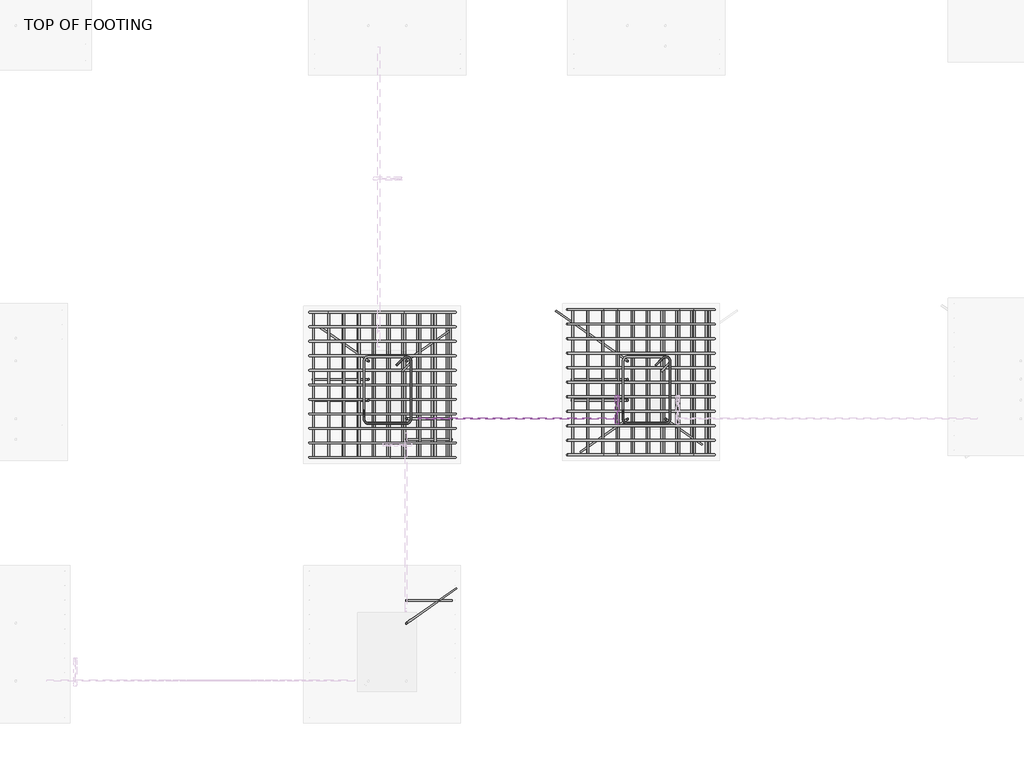
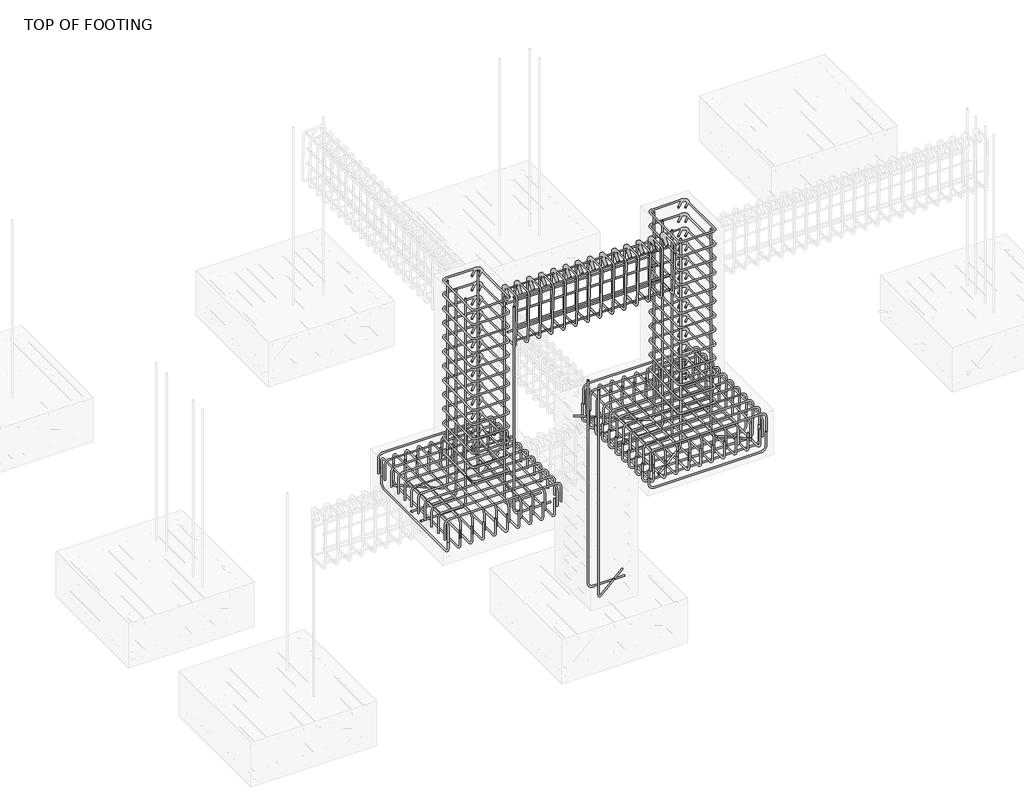
# One storey, part 4 of 17: 24 reinforcing bars.
"""IFC4 building model written with IfcOpenShell, lengths in millimetres."""

from ifc_helpers import new_model, si_unit, point, frame, origin, place, context, project, spatial, polyline, circle_curve, trimmed, segment, composite_curve, source, transform, mapped, element, save
from ifc_brep_helpers import swept_disk

model = new_model("IFC4")

# Units and contexts
model_context = context("Model", 3, world=origin())
ifc_project = project(units=[si_unit("LENGTHUNIT", "METRE", prefix="MILLI")], contexts=[model_context])

# Site, building, storey
site = spatial("IfcSite", under=ifc_project)
building = spatial("IfcBuilding", under=site)
storey = spatial("IfcBuildingStorey", under=building, Name="TOP OF FOOTING", Elevation=-1828.8)

# Reinforcing bars
placement = place(None, origin())
reinforcing_bar_shape = source(origin(), model_context, "Body", "SolidModel", [
    swept_disk(composite_curve([segment(polyline([(-908.0711351, -340.8742842, -2058.517229), (-908.0711351, -340.8742842, -1911.217229)]), True, "CONTINUOUS"), segment(trimmed(circle_curve(frame((-861.7211351, -340.8742842, -1911.217229), z_axis=(0.0, 1.0, 0.0), x_axis=(-46.35000000000002, 0.0, 0.0)), 46.35), [point((-908.0711351, -340.8742842, -1911.217229))], [point((-861.7211351, -340.8742842, -1864.867229))], True, "CARTESIAN"), True, "CONTINUOUS"), segment(polyline([(-861.7211351, -340.8742842, -1864.867229), (156.8352514, -340.8742842, -1864.867229)]), True, "CONTINUOUS"), segment(trimmed(circle_curve(frame((156.8352514, -340.8742842, -1911.217229), z_axis=(0.0, 1.0, 0.0), x_axis=(0.0, 0.0, 46.350000000000136)), 46.35), [point((156.8352514, -340.8742842, -1864.867229))], [point((203.1852514, -340.8742842, -1911.217229))], True, "CARTESIAN"), True, "CONTINUOUS"), segment(polyline([(203.1852514, -340.8742842, -1911.217229), (203.1852514, -340.8742842, -2058.517229)]), True, "CONTINUOUS")], self_intersect=False), 6.35),
])
element("IfcReinforcingBar", 1, at=placement, inside=storey, context=model_context, shape_type="MappedRepresentation", body=[
    mapped(reinforcing_bar_shape, transform((0.0, 0.0, 0.0), x_axis=(1.0, 0.0, 0.0), y_axis=(0.0, 1.0, 0.0), z_axis=(0.0, 0.0, 1.0))),
    mapped(reinforcing_bar_shape, transform((0.0, -110.73, 0.0), x_axis=(1.0, 0.0, 0.0), y_axis=(0.0, 1.0, 0.0), z_axis=(0.0, 0.0, 1.0))),
    mapped(reinforcing_bar_shape, transform((0.0, -221.46, 0.0), x_axis=(1.0, 0.0, 0.0), y_axis=(0.0, 1.0, 0.0), z_axis=(0.0, 0.0, 1.0))),
    mapped(reinforcing_bar_shape, transform((0.0, -332.19, 0.0), x_axis=(1.0, 0.0, 0.0), y_axis=(0.0, 1.0, 0.0), z_axis=(0.0, 0.0, 1.0))),
    mapped(reinforcing_bar_shape, transform((0.0, -442.92, 0.0), x_axis=(1.0, 0.0, 0.0), y_axis=(0.0, 1.0, 0.0), z_axis=(0.0, 0.0, 1.0))),
    mapped(reinforcing_bar_shape, transform((0.0, -553.65, 0.0), x_axis=(1.0, 0.0, 0.0), y_axis=(0.0, 1.0, 0.0), z_axis=(0.0, 0.0, 1.0))),
    mapped(reinforcing_bar_shape, transform((0.0, -664.38, 0.0), x_axis=(1.0, 0.0, 0.0), y_axis=(0.0, 1.0, 0.0), z_axis=(0.0, 0.0, 1.0))),
    mapped(reinforcing_bar_shape, transform((0.0, -775.11, 0.0), x_axis=(1.0, 0.0, 0.0), y_axis=(0.0, 1.0, 0.0), z_axis=(0.0, 0.0, 1.0))),
    mapped(reinforcing_bar_shape, transform((0.0, -885.84, 0.0), x_axis=(1.0, 0.0, 0.0), y_axis=(0.0, 1.0, 0.0), z_axis=(0.0, 0.0, 1.0))),
    mapped(reinforcing_bar_shape, transform((0.0, -996.57, 0.0), x_axis=(1.0, 0.0, 0.0), y_axis=(0.0, 1.0, 0.0), z_axis=(0.0, 0.0, 1.0))),
    mapped(reinforcing_bar_shape, transform((0.0, -1107.3, 0.0), x_axis=(1.0, 0.0, 0.0), y_axis=(0.0, 1.0, 0.0), z_axis=(0.0, 0.0, 1.0))),
])
reinforcing_bar_2_shape = source(origin(), model_context, "Body", "SolidModel", [
    swept_disk(composite_curve([segment(polyline([(166.1935463, -340.8742842, -2093.0974099), (166.1935463, -340.8742842, -1945.7974099)]), True, "CONTINUOUS"), segment(trimmed(circle_curve(frame((166.1935463, -387.2242842, -1945.7974099), z_axis=(1.0, 0.0, 0.0), x_axis=(0.0, 46.35000000000002, 0.0)), 46.35), [point((166.1935463, -340.8742842, -1945.7974099))], [point((166.1935463, -387.2242842, -1899.4474099))], True, "CARTESIAN"), True, "CONTINUOUS"), segment(polyline([(166.1935463, -387.2242842, -1899.4474099), (166.1935463, -1401.8242842, -1899.4474099)]), True, "CONTINUOUS"), segment(trimmed(circle_curve(frame((166.1935463, -1401.8242842, -1945.7974099), z_axis=(1.0, 0.0, 0.0), x_axis=(0.0, 0.0, 46.350000000000136)), 46.35), [point((166.1935463, -1401.8242842, -1899.4474099))], [point((166.1935463, -1448.1742842, -1945.7974099))], True, "CARTESIAN"), True, "CONTINUOUS"), segment(polyline([(166.1935463, -1448.1742842, -1945.7974099), (166.1935463, -1448.1742842, -2093.0974099)]), True, "CONTINUOUS")], self_intersect=False), 6.35),
])
element("IfcReinforcingBar", 2, at=placement, inside=storey, context=model_context, shape_type="MappedRepresentation", body=[
    mapped(reinforcing_bar_2_shape, transform((0.0, 0.0, 0.0), x_axis=(1.0, 0.0, 0.0), y_axis=(0.0, 1.0, 0.0), z_axis=(0.0, 0.0, 1.0))),
    mapped(reinforcing_bar_2_shape, transform((-115.9606781, 0.0, 0.0), x_axis=(1.0, 0.0, 0.0), y_axis=(0.0, 1.0, 0.0), z_axis=(0.0, 0.0, 1.0))),
    mapped(reinforcing_bar_2_shape, transform((-231.9213561, 0.0, 0.0), x_axis=(1.0, 0.0, 0.0), y_axis=(0.0, 1.0, 0.0), z_axis=(0.0, 0.0, 1.0))),
    mapped(reinforcing_bar_2_shape, transform((-347.8820342, 0.0, 0.0), x_axis=(1.0, 0.0, 0.0), y_axis=(0.0, 1.0, 0.0), z_axis=(0.0, 0.0, 1.0))),
    mapped(reinforcing_bar_2_shape, transform((-463.8427123, 0.0, 0.0), x_axis=(1.0, 0.0, 0.0), y_axis=(0.0, 1.0, 0.0), z_axis=(0.0, 0.0, 1.0))),
    mapped(reinforcing_bar_2_shape, transform((-579.8033904, 0.0, 0.0), x_axis=(1.0, 0.0, 0.0), y_axis=(0.0, 1.0, 0.0), z_axis=(0.0, 0.0, 1.0))),
    mapped(reinforcing_bar_2_shape, transform((-695.7640684, 0.0, 0.0), x_axis=(1.0, 0.0, 0.0), y_axis=(0.0, 1.0, 0.0), z_axis=(0.0, 0.0, 1.0))),
    mapped(reinforcing_bar_2_shape, transform((-811.7247465, 0.0, 0.0), x_axis=(1.0, 0.0, 0.0), y_axis=(0.0, 1.0, 0.0), z_axis=(0.0, 0.0, 1.0))),
    mapped(reinforcing_bar_2_shape, transform((-927.6854246, 0.0, 0.0), x_axis=(1.0, 0.0, 0.0), y_axis=(0.0, 1.0, 0.0), z_axis=(0.0, 0.0, 1.0))),
    mapped(reinforcing_bar_2_shape, transform((-1043.6461027, 0.0, 0.0), x_axis=(1.0, 0.0, 0.0), y_axis=(0.0, 1.0, 0.0), z_axis=(0.0, 0.0, 1.0))),
])
reinforcing_bar_3_shape = source(origin(), model_context, "Body", "SolidModel", [
    swept_disk(composite_curve([segment(polyline([(-877.4525564, -340.8742842, -2009.4698822), (-877.4525564, -340.8742842, -2156.7698822)]), True, "CONTINUOUS"), segment(trimmed(circle_curve(frame((-877.4525564, -387.2242842, -2156.7698822), z_axis=(-1.0, 0.0, 0.0), x_axis=(0.0, 46.35000000000002, 0.0)), 46.35), [point((-877.4525564, -340.8742842, -2156.7698822))], [point((-877.4525564, -387.2242842, -2203.1198822))], True, "CARTESIAN"), True, "CONTINUOUS"), segment(polyline([(-877.4525564, -387.2242842, -2203.1198822), (-877.4525564, -1401.8242842, -2203.1198822)]), True, "CONTINUOUS"), segment(trimmed(circle_curve(frame((-877.4525564, -1401.8242842, -2156.7698822), z_axis=(-1.0, 0.0, 0.0), x_axis=(0.0, 0.0, -46.34999999999991)), 46.35), [point((-877.4525564, -1401.8242842, -2203.1198822))], [point((-877.4525564, -1448.1742842, -2156.7698822))], True, "CARTESIAN"), True, "CONTINUOUS"), segment(polyline([(-877.4525564, -1448.1742842, -2156.7698822), (-877.4525564, -1448.1742842, -2009.4698822)]), True, "CONTINUOUS")], self_intersect=False), 6.35),
])
element("IfcReinforcingBar", 3, at=placement, inside=storey, context=model_context, shape_type="MappedRepresentation", body=[
    mapped(reinforcing_bar_3_shape, transform((0.0, 0.0, 0.0), x_axis=(1.0, 0.0, 0.0), y_axis=(0.0, 1.0, 0.0), z_axis=(0.0, 0.0, 1.0))),
    mapped(reinforcing_bar_3_shape, transform((113.1523491, 0.0, 0.0), x_axis=(1.0, 0.0, 0.0), y_axis=(0.0, 1.0, 0.0), z_axis=(0.0, 0.0, 1.0))),
    mapped(reinforcing_bar_3_shape, transform((226.3046983, 0.0, 0.0), x_axis=(1.0, 0.0, 0.0), y_axis=(0.0, 1.0, 0.0), z_axis=(0.0, 0.0, 1.0))),
    mapped(reinforcing_bar_3_shape, transform((339.4570474, 0.0, 0.0), x_axis=(1.0, 0.0, 0.0), y_axis=(0.0, 1.0, 0.0), z_axis=(0.0, 0.0, 1.0))),
    mapped(reinforcing_bar_3_shape, transform((452.6093966, 0.0, 0.0), x_axis=(1.0, 0.0, 0.0), y_axis=(0.0, 1.0, 0.0), z_axis=(0.0, 0.0, 1.0))),
    mapped(reinforcing_bar_3_shape, transform((565.7617457, 0.0, 0.0), x_axis=(1.0, 0.0, 0.0), y_axis=(0.0, 1.0, 0.0), z_axis=(0.0, 0.0, 1.0))),
    mapped(reinforcing_bar_3_shape, transform((678.9140949, 0.0, 0.0), x_axis=(1.0, 0.0, 0.0), y_axis=(0.0, 1.0, 0.0), z_axis=(0.0, 0.0, 1.0))),
    mapped(reinforcing_bar_3_shape, transform((792.066444, 0.0, 0.0), x_axis=(1.0, 0.0, 0.0), y_axis=(0.0, 1.0, 0.0), z_axis=(0.0, 0.0, 1.0))),
    mapped(reinforcing_bar_3_shape, transform((905.2187932, 0.0, 0.0), x_axis=(1.0, 0.0, 0.0), y_axis=(0.0, 1.0, 0.0), z_axis=(0.0, 0.0, 1.0))),
    mapped(reinforcing_bar_3_shape, transform((1018.3711423, 0.0, 0.0), x_axis=(1.0, 0.0, 0.0), y_axis=(0.0, 1.0, 0.0), z_axis=(0.0, 0.0, 1.0))),
])
reinforcing_bar_4_shape = source(origin(), model_context, "Body", "SolidModel", [
    swept_disk(composite_curve([segment(polyline([(2175.7588658, -320.8742842, -2051.4362487), (2175.7588658, -320.8742842, -2198.7362487)]), True, "CONTINUOUS"), segment(trimmed(circle_curve(frame((2129.4088658, -320.8742842, -2198.7362487), z_axis=(0.0, 1.0, 0.0), x_axis=(46.34999999999991, 0.0, 0.0)), 46.35), [point((2175.7588658, -320.8742842, -2198.7362487))], [point((2129.4088658, -320.8742842, -2245.0862487))], True, "CARTESIAN"), True, "CONTINUOUS"), segment(polyline([(2129.4088658, -320.8742842, -2245.0862487), (1104.0910413, -320.8742842, -2245.0862487)]), True, "CONTINUOUS"), segment(trimmed(circle_curve(frame((1104.0910413, -320.8742842, -2198.7362487), z_axis=(0.0, 1.0, 0.0), x_axis=(0.0, 0.0, -46.34999999999991)), 46.35), [point((1104.0910413, -320.8742842, -2245.0862487))], [point((1057.7410413, -320.8742842, -2198.7362487))], True, "CARTESIAN"), True, "CONTINUOUS"), segment(polyline([(1057.7410413, -320.8742842, -2198.7362487), (1057.7410413, -320.8742842, -2051.4362487)]), True, "CONTINUOUS")], self_intersect=False), 6.35),
])
element("IfcReinforcingBar", 4, at=placement, inside=storey, context=model_context, shape_type="MappedRepresentation", body=[
    mapped(reinforcing_bar_4_shape, transform((0.0, 0.0, 0.0), x_axis=(1.0, 0.0, 0.0), y_axis=(0.0, 1.0, 0.0), z_axis=(0.0, 0.0, 1.0))),
    mapped(reinforcing_bar_4_shape, transform((0.0, -110.73, 0.0), x_axis=(1.0, 0.0, 0.0), y_axis=(0.0, 1.0, 0.0), z_axis=(0.0, 0.0, 1.0))),
    mapped(reinforcing_bar_4_shape, transform((0.0, -221.46, 0.0), x_axis=(1.0, 0.0, 0.0), y_axis=(0.0, 1.0, 0.0), z_axis=(0.0, 0.0, 1.0))),
    mapped(reinforcing_bar_4_shape, transform((0.0, -332.19, 0.0), x_axis=(1.0, 0.0, 0.0), y_axis=(0.0, 1.0, 0.0), z_axis=(0.0, 0.0, 1.0))),
    mapped(reinforcing_bar_4_shape, transform((0.0, -442.92, 0.0), x_axis=(1.0, 0.0, 0.0), y_axis=(0.0, 1.0, 0.0), z_axis=(0.0, 0.0, 1.0))),
    mapped(reinforcing_bar_4_shape, transform((0.0, -553.65, 0.0), x_axis=(1.0, 0.0, 0.0), y_axis=(0.0, 1.0, 0.0), z_axis=(0.0, 0.0, 1.0))),
    mapped(reinforcing_bar_4_shape, transform((0.0, -664.38, 0.0), x_axis=(1.0, 0.0, 0.0), y_axis=(0.0, 1.0, 0.0), z_axis=(0.0, 0.0, 1.0))),
    mapped(reinforcing_bar_4_shape, transform((0.0, -775.11, 0.0), x_axis=(1.0, 0.0, 0.0), y_axis=(0.0, 1.0, 0.0), z_axis=(0.0, 0.0, 1.0))),
    mapped(reinforcing_bar_4_shape, transform((0.0, -885.84, 0.0), x_axis=(1.0, 0.0, 0.0), y_axis=(0.0, 1.0, 0.0), z_axis=(0.0, 0.0, 1.0))),
    mapped(reinforcing_bar_4_shape, transform((0.0, -996.57, 0.0), x_axis=(1.0, 0.0, 0.0), y_axis=(0.0, 1.0, 0.0), z_axis=(0.0, 0.0, 1.0))),
    mapped(reinforcing_bar_4_shape, transform((0.0, -1107.3, 0.0), x_axis=(1.0, 0.0, 0.0), y_axis=(0.0, 1.0, 0.0), z_axis=(0.0, 0.0, 1.0))),
])
reinforcing_bar_5_shape = source(origin(), model_context, "Body", "SolidModel", [
    swept_disk(composite_curve([segment(polyline([(1068.404705, -320.8742842, -2058.517229), (1068.404705, -320.8742842, -1911.217229)]), True, "CONTINUOUS"), segment(trimmed(circle_curve(frame((1114.754705, -320.8742842, -1911.217229), z_axis=(0.0, 1.0, 0.0), x_axis=(-46.350000000000136, 0.0, 0.0)), 46.35), [point((1068.404705, -320.8742842, -1911.217229))], [point((1114.754705, -320.8742842, -1864.867229))], True, "CARTESIAN"), True, "CONTINUOUS"), segment(polyline([(1114.754705, -320.8742842, -1864.867229), (2133.3110915, -320.8742842, -1864.867229)]), True, "CONTINUOUS"), segment(trimmed(circle_curve(frame((2133.3110915, -320.8742842, -1911.217229), z_axis=(0.0, 1.0, 0.0), x_axis=(0.0, 0.0, 46.350000000000136)), 46.35), [point((2133.3110915, -320.8742842, -1864.867229))], [point((2179.6610915, -320.8742842, -1911.217229))], True, "CARTESIAN"), True, "CONTINUOUS"), segment(polyline([(2179.6610915, -320.8742842, -1911.217229), (2179.6610915, -320.8742842, -2058.517229)]), True, "CONTINUOUS")], self_intersect=False), 6.35),
])
element("IfcReinforcingBar", 5, at=placement, inside=storey, context=model_context, shape_type="MappedRepresentation", body=[
    mapped(reinforcing_bar_5_shape, transform((0.0, 0.0, 0.0), x_axis=(1.0, 0.0, 0.0), y_axis=(0.0, 1.0, 0.0), z_axis=(0.0, 0.0, 1.0))),
    mapped(reinforcing_bar_5_shape, transform((0.0, -110.73, 0.0), x_axis=(1.0, 0.0, 0.0), y_axis=(0.0, 1.0, 0.0), z_axis=(0.0, 0.0, 1.0))),
    mapped(reinforcing_bar_5_shape, transform((0.0, -221.46, 0.0), x_axis=(1.0, 0.0, 0.0), y_axis=(0.0, 1.0, 0.0), z_axis=(0.0, 0.0, 1.0))),
    mapped(reinforcing_bar_5_shape, transform((0.0, -332.19, 0.0), x_axis=(1.0, 0.0, 0.0), y_axis=(0.0, 1.0, 0.0), z_axis=(0.0, 0.0, 1.0))),
    mapped(reinforcing_bar_5_shape, transform((0.0, -442.92, 0.0), x_axis=(1.0, 0.0, 0.0), y_axis=(0.0, 1.0, 0.0), z_axis=(0.0, 0.0, 1.0))),
    mapped(reinforcing_bar_5_shape, transform((0.0, -553.65, 0.0), x_axis=(1.0, 0.0, 0.0), y_axis=(0.0, 1.0, 0.0), z_axis=(0.0, 0.0, 1.0))),
    mapped(reinforcing_bar_5_shape, transform((0.0, -664.38, 0.0), x_axis=(1.0, 0.0, 0.0), y_axis=(0.0, 1.0, 0.0), z_axis=(0.0, 0.0, 1.0))),
    mapped(reinforcing_bar_5_shape, transform((0.0, -775.11, 0.0), x_axis=(1.0, 0.0, 0.0), y_axis=(0.0, 1.0, 0.0), z_axis=(0.0, 0.0, 1.0))),
    mapped(reinforcing_bar_5_shape, transform((0.0, -885.84, 0.0), x_axis=(1.0, 0.0, 0.0), y_axis=(0.0, 1.0, 0.0), z_axis=(0.0, 0.0, 1.0))),
    mapped(reinforcing_bar_5_shape, transform((0.0, -996.57, 0.0), x_axis=(1.0, 0.0, 0.0), y_axis=(0.0, 1.0, 0.0), z_axis=(0.0, 0.0, 1.0))),
    mapped(reinforcing_bar_5_shape, transform((0.0, -1107.3, 0.0), x_axis=(1.0, 0.0, 0.0), y_axis=(0.0, 1.0, 0.0), z_axis=(0.0, 0.0, 1.0))),
])
reinforcing_bar_6_shape = source(origin(), model_context, "Body", "SolidModel", [
    swept_disk(composite_curve([segment(polyline([(2142.6693864, -320.8742842, -2093.0974099), (2142.6693864, -320.8742842, -1945.7974099)]), True, "CONTINUOUS"), segment(trimmed(circle_curve(frame((2142.6693864, -367.2242842, -1945.7974099), z_axis=(1.0, 0.0, 0.0), x_axis=(0.0, 46.35000000000002, 0.0)), 46.35), [point((2142.6693864, -320.8742842, -1945.7974099))], [point((2142.6693864, -367.2242842, -1899.4474099))], True, "CARTESIAN"), True, "CONTINUOUS"), segment(polyline([(2142.6693864, -367.2242842, -1899.4474099), (2142.6693864, -1381.8242842, -1899.4474099)]), True, "CONTINUOUS"), segment(trimmed(circle_curve(frame((2142.6693864, -1381.8242842, -1945.7974099), z_axis=(1.0, 0.0, 0.0), x_axis=(0.0, 0.0, 46.350000000000136)), 46.35), [point((2142.6693864, -1381.8242842, -1899.4474099))], [point((2142.6693864, -1428.1742842, -1945.7974099))], True, "CARTESIAN"), True, "CONTINUOUS"), segment(polyline([(2142.6693864, -1428.1742842, -1945.7974099), (2142.6693864, -1428.1742842, -2093.0974099)]), True, "CONTINUOUS")], self_intersect=False), 6.35),
])
element("IfcReinforcingBar", 6, at=placement, inside=storey, context=model_context, shape_type="MappedRepresentation", body=[
    mapped(reinforcing_bar_6_shape, transform((0.0, 0.0, 0.0), x_axis=(1.0, 0.0, 0.0), y_axis=(0.0, 1.0, 0.0), z_axis=(0.0, 0.0, 1.0))),
    mapped(reinforcing_bar_6_shape, transform((-115.9606781, 0.0, 0.0), x_axis=(1.0, 0.0, 0.0), y_axis=(0.0, 1.0, 0.0), z_axis=(0.0, 0.0, 1.0))),
    mapped(reinforcing_bar_6_shape, transform((-231.9213561, 0.0, 0.0), x_axis=(1.0, 0.0, 0.0), y_axis=(0.0, 1.0, 0.0), z_axis=(0.0, 0.0, 1.0))),
    mapped(reinforcing_bar_6_shape, transform((-347.8820342, 0.0, 0.0), x_axis=(1.0, 0.0, 0.0), y_axis=(0.0, 1.0, 0.0), z_axis=(0.0, 0.0, 1.0))),
    mapped(reinforcing_bar_6_shape, transform((-463.8427123, 0.0, 0.0), x_axis=(1.0, 0.0, 0.0), y_axis=(0.0, 1.0, 0.0), z_axis=(0.0, 0.0, 1.0))),
    mapped(reinforcing_bar_6_shape, transform((-579.8033904, 0.0, 0.0), x_axis=(1.0, 0.0, 0.0), y_axis=(0.0, 1.0, 0.0), z_axis=(0.0, 0.0, 1.0))),
    mapped(reinforcing_bar_6_shape, transform((-695.7640684, 0.0, 0.0), x_axis=(1.0, 0.0, 0.0), y_axis=(0.0, 1.0, 0.0), z_axis=(0.0, 0.0, 1.0))),
    mapped(reinforcing_bar_6_shape, transform((-811.7247465, 0.0, 0.0), x_axis=(1.0, 0.0, 0.0), y_axis=(0.0, 1.0, 0.0), z_axis=(0.0, 0.0, 1.0))),
    mapped(reinforcing_bar_6_shape, transform((-927.6854246, 0.0, 0.0), x_axis=(1.0, 0.0, 0.0), y_axis=(0.0, 1.0, 0.0), z_axis=(0.0, 0.0, 1.0))),
    mapped(reinforcing_bar_6_shape, transform((-1043.6461027, 0.0, 0.0), x_axis=(1.0, 0.0, 0.0), y_axis=(0.0, 1.0, 0.0), z_axis=(0.0, 0.0, 1.0))),
])
reinforcing_bar_7_shape = source(origin(), model_context, "Body", "SolidModel", [
    swept_disk(composite_curve([segment(polyline([(1099.0232837, -320.8742842, -2009.4698822), (1099.0232837, -320.8742842, -2156.7698822)]), True, "CONTINUOUS"), segment(trimmed(circle_curve(frame((1099.0232837, -367.2242842, -2156.7698822), z_axis=(-1.0, 0.0, 0.0), x_axis=(0.0, 46.35000000000002, 0.0)), 46.35), [point((1099.0232837, -320.8742842, -2156.7698822))], [point((1099.0232837, -367.2242842, -2203.1198822))], True, "CARTESIAN"), True, "CONTINUOUS"), segment(polyline([(1099.0232837, -367.2242842, -2203.1198822), (1099.0232837, -1381.8242842, -2203.1198822)]), True, "CONTINUOUS"), segment(trimmed(circle_curve(frame((1099.0232837, -1381.8242842, -2156.7698822), z_axis=(-1.0, 0.0, 0.0), x_axis=(0.0, 0.0, -46.34999999999991)), 46.35), [point((1099.0232837, -1381.8242842, -2203.1198822))], [point((1099.0232837, -1428.1742842, -2156.7698822))], True, "CARTESIAN"), True, "CONTINUOUS"), segment(polyline([(1099.0232837, -1428.1742842, -2156.7698822), (1099.0232837, -1428.1742842, -2009.4698822)]), True, "CONTINUOUS")], self_intersect=False), 6.35),
])
element("IfcReinforcingBar", 7, at=placement, inside=storey, context=model_context, shape_type="MappedRepresentation", body=[
    mapped(reinforcing_bar_7_shape, transform((0.0, 0.0, 0.0), x_axis=(1.0, 0.0, 0.0), y_axis=(0.0, 1.0, 0.0), z_axis=(0.0, 0.0, 1.0))),
    mapped(reinforcing_bar_7_shape, transform((113.1523491, 0.0, 0.0), x_axis=(1.0, 0.0, 0.0), y_axis=(0.0, 1.0, 0.0), z_axis=(0.0, 0.0, 1.0))),
    mapped(reinforcing_bar_7_shape, transform((226.3046983, 0.0, 0.0), x_axis=(1.0, 0.0, 0.0), y_axis=(0.0, 1.0, 0.0), z_axis=(0.0, 0.0, 1.0))),
    mapped(reinforcing_bar_7_shape, transform((339.4570474, 0.0, 0.0), x_axis=(1.0, 0.0, 0.0), y_axis=(0.0, 1.0, 0.0), z_axis=(0.0, 0.0, 1.0))),
    mapped(reinforcing_bar_7_shape, transform((452.6093966, 0.0, 0.0), x_axis=(1.0, 0.0, 0.0), y_axis=(0.0, 1.0, 0.0), z_axis=(0.0, 0.0, 1.0))),
    mapped(reinforcing_bar_7_shape, transform((565.7617457, 0.0, 0.0), x_axis=(1.0, 0.0, 0.0), y_axis=(0.0, 1.0, 0.0), z_axis=(0.0, 0.0, 1.0))),
    mapped(reinforcing_bar_7_shape, transform((678.9140949, 0.0, 0.0), x_axis=(1.0, 0.0, 0.0), y_axis=(0.0, 1.0, 0.0), z_axis=(0.0, 0.0, 1.0))),
    mapped(reinforcing_bar_7_shape, transform((792.066444, 0.0, 0.0), x_axis=(1.0, 0.0, 0.0), y_axis=(0.0, 1.0, 0.0), z_axis=(0.0, 0.0, 1.0))),
    mapped(reinforcing_bar_7_shape, transform((905.2187932, 0.0, 0.0), x_axis=(1.0, 0.0, 0.0), y_axis=(0.0, 1.0, 0.0), z_axis=(0.0, 0.0, 1.0))),
    mapped(reinforcing_bar_7_shape, transform((1018.3711423, 0.0, 0.0), x_axis=(1.0, 0.0, 0.0), y_axis=(0.0, 1.0, 0.0), z_axis=(0.0, 0.0, 1.0))),
])
reinforcing_bar_8_shape = source(origin(), model_context, "Body", "SolidModel", [
    swept_disk(composite_curve([segment(polyline([(-170.102564, -2539.9309999, -40.0), (-170.102564, -2539.9309999, -2094.5391135)]), True, "CONTINUOUS"), segment(trimmed(circle_curve(frame((-123.752564, -2539.9309999, -2094.5391135), z_axis=(0.0, -1.0, 0.0), x_axis=(-46.349999999999994, 0.0, 0.0)), 46.35), [point((-170.102564, -2539.9309999, -2094.5391135))], [point((-123.752564, -2539.9309999, -2140.8891135))], True, "CARTESIAN"), True, "CONTINUOUS"), segment(polyline([(-123.752564, -2539.9309999, -2140.8891135), (179.9793434, -2539.9309999, -2140.8891135)]), True, "CONTINUOUS")], self_intersect=False), 6.35),
])
element("IfcReinforcingBar", 8, at=placement, inside=storey, context=model_context, shape_type="MappedRepresentation", body=[
    mapped(reinforcing_bar_8_shape, transform((0.0, 0.0, 0.0), x_axis=(1.0, 0.0, 0.0), y_axis=(0.0, 1.0, 0.0), z_axis=(0.0, 0.0, 1.0))),
    mapped(reinforcing_bar_8_shape, transform((0.0, 1228.0260466, 0.0), x_axis=(1.0, 0.0, 0.0), y_axis=(0.0, 1.0, 0.0), z_axis=(0.0, 0.0, 1.0))),
])
element("IfcReinforcingBar", 9, at=placement, inside=storey, context=model_context, shape_type="SolidModel", body=[
    swept_disk(composite_curve([segment(polyline([(-170.102564, -2713.5742842, -40.0), (-170.102564, -2713.5742842, -2094.5391135)]), True, "CONTINUOUS"), segment(trimmed(circle_curve(frame((-132.1348667, -2686.9890164, -2094.5391135), z_axis=(0.5735764363510363, -0.8191520442889988, 0.0), x_axis=(-37.9676973, -26.58526780000011, 0.0)), 46.35), [point((-170.102564, -2713.5742842, -2094.5391135))], [point((-132.1348667, -2686.9890164, -2140.8891135))], True, "CARTESIAN"), True, "CONTINUOUS"), segment(polyline([(-132.1348667, -2686.9890164, -2140.8891135), (212.5638338, -2445.6283879, -2140.8891135)]), True, "CONTINUOUS")], self_intersect=False), 6.35),
])
reinforcing_bar_9_shape = source(origin(), model_context, "Body", "SolidModel", [
    swept_disk(composite_curve([segment(polyline([(-244.9783349, -745.8000495, -46.35), (-189.2347719, -690.0564866, -46.35)]), True, "CONTINUOUS"), segment(trimmed(circle_curve(frame((-167.0669743, -712.2242842, -46.35), z_axis=(0.0, 0.0, -1.0), x_axis=(-22.1677976, 22.167797600000085, 0.0)), 31.35), [point((-189.2347719, -690.0564866, -46.35))], [point((-135.7169743, -712.2242842, -46.35))], True, "CARTESIAN"), True, "CONTINUOUS"), segment(polyline([(-135.7169743, -712.2242842, -46.35), (-135.7169743, -1156.8242842, -46.35)]), True, "CONTINUOUS"), segment(trimmed(circle_curve(frame((-167.0669743, -1156.8242842, -46.35), z_axis=(0.0, 0.0, -1.0), x_axis=(31.349999999999994, 0.0, 0.0)), 31.35), [point((-135.7169743, -1156.8242842, -46.35))], [point((-167.0669743, -1188.1742842, -46.35))], True, "CARTESIAN"), True, "CONTINUOUS"), segment(polyline([(-167.0669743, -1188.1742842, -46.35), (-461.6669743, -1188.1742842, -46.35)]), True, "CONTINUOUS"), segment(trimmed(circle_curve(frame((-461.6669743, -1156.8341035, -45.5654144), z_axis=(0.0, 0.025026655153786343, -0.9996867842138424), x_axis=(0.0, -31.34018070000002, -0.7845855999999998)), 31.35), [point((-461.6669743, -1188.1742842, -46.35))], [point((-493.0169743, -1156.8341035, -45.5654144))], True, "CARTESIAN"), True, "CONTINUOUS"), segment(polyline([(-493.0169743, -1156.8341035, -45.5654144), (-493.0169743, -712.2144649, -34.4345856)]), True, "CONTINUOUS"), segment(trimmed(circle_curve(frame((-461.6669743, -712.2144649, -34.4345856), z_axis=(0.0, 0.025026655153786343, -0.9996867842138424), x_axis=(-31.350000000000023, 0.0, 0.0)), 31.35), [point((-493.0169743, -712.2144649, -34.4345856))], [point((-461.6669743, -680.8742842, -33.65))], True, "CARTESIAN"), True, "CONTINUOUS"), segment(polyline([(-461.6669743, -680.8742842, -33.65), (-167.0669743, -680.8742842, -33.65)]), True, "CONTINUOUS"), segment(trimmed(circle_curve(frame((-167.0669743, -712.2242842, -33.65), z_axis=(0.0, 0.0, -1.0), x_axis=(0.0, 31.350000000000023, 0.0)), 31.35), [point((-167.0669743, -680.8742842, -33.65))], [point((-144.8991767, -734.3920818, -33.65))], True, "CARTESIAN"), True, "CONTINUOUS"), segment(polyline([(-144.8991767, -734.3920818, -33.65), (-200.6427397, -790.1356447, -33.65)]), True, "CONTINUOUS")], self_intersect=False), 6.35),
])
element("IfcReinforcingBar", 10, at=placement, inside=storey, context=model_context, shape_type="MappedRepresentation", body=[
    mapped(reinforcing_bar_9_shape, transform((0.0, 0.0, 0.0), x_axis=(1.0, 0.0, 0.0), y_axis=(0.0, 1.0, 0.0), z_axis=(0.0, 0.0, 1.0))),
    mapped(reinforcing_bar_9_shape, transform((0.0, 0.0, -144.675), x_axis=(1.0, 0.0, 0.0), y_axis=(0.0, 1.0, 0.0), z_axis=(0.0, 0.0, 1.0))),
    mapped(reinforcing_bar_9_shape, transform((0.0, 0.0, -289.35), x_axis=(1.0, 0.0, 0.0), y_axis=(0.0, 1.0, 0.0), z_axis=(0.0, 0.0, 1.0))),
    mapped(reinforcing_bar_9_shape, transform((0.0, 0.0, -434.025), x_axis=(1.0, 0.0, 0.0), y_axis=(0.0, 1.0, 0.0), z_axis=(0.0, 0.0, 1.0))),
    mapped(reinforcing_bar_9_shape, transform((0.0, 0.0, -578.7), x_axis=(1.0, 0.0, 0.0), y_axis=(0.0, 1.0, 0.0), z_axis=(0.0, 0.0, 1.0))),
    mapped(reinforcing_bar_9_shape, transform((0.0, 0.0, -723.375), x_axis=(1.0, 0.0, 0.0), y_axis=(0.0, 1.0, 0.0), z_axis=(0.0, 0.0, 1.0))),
    mapped(reinforcing_bar_9_shape, transform((0.0, 0.0, -868.05), x_axis=(1.0, 0.0, 0.0), y_axis=(0.0, 1.0, 0.0), z_axis=(0.0, 0.0, 1.0))),
    mapped(reinforcing_bar_9_shape, transform((0.0, 0.0, -1012.725), x_axis=(1.0, 0.0, 0.0), y_axis=(0.0, 1.0, 0.0), z_axis=(0.0, 0.0, 1.0))),
    mapped(reinforcing_bar_9_shape, transform((0.0, 0.0, -1157.4), x_axis=(1.0, 0.0, 0.0), y_axis=(0.0, 1.0, 0.0), z_axis=(0.0, 0.0, 1.0))),
    mapped(reinforcing_bar_9_shape, transform((0.0, 0.0, -1302.075), x_axis=(1.0, 0.0, 0.0), y_axis=(0.0, 1.0, 0.0), z_axis=(0.0, 0.0, 1.0))),
    mapped(reinforcing_bar_9_shape, transform((0.0, 0.0, -1446.75), x_axis=(1.0, 0.0, 0.0), y_axis=(0.0, 1.0, 0.0), z_axis=(0.0, 0.0, 1.0))),
    mapped(reinforcing_bar_9_shape, transform((0.0, 0.0, -1591.425), x_axis=(1.0, 0.0, 0.0), y_axis=(0.0, 1.0, 0.0), z_axis=(0.0, 0.0, 1.0))),
    mapped(reinforcing_bar_9_shape, transform((0.0, 0.0, -1736.1), x_axis=(1.0, 0.0, 0.0), y_axis=(0.0, 1.0, 0.0), z_axis=(0.0, 0.0, 1.0))),
])
reinforcing_bar_10_shape = source(origin(), model_context, "Body", "SolidModel", [
    swept_disk(composite_curve([segment(polyline([(-170.102564, -1152.6310005, -40.0), (-170.102564, -1152.6310005, -2094.5391135)]), True, "CONTINUOUS"), segment(trimmed(circle_curve(frame((-123.752564, -1152.6310005, -2094.5391135), z_axis=(0.0, -1.0, 0.0), x_axis=(-46.349999999999994, 0.0, 0.0)), 46.35), [point((-170.102564, -1152.6310005, -2094.5391135))], [point((-123.752564, -1152.6310005, -2140.8891135))], True, "CARTESIAN"), True, "CONTINUOUS"), segment(polyline([(-123.752564, -1152.6310005, -2140.8891135), (179.9793434, -1152.6310005, -2140.8891135)]), True, "CONTINUOUS")], self_intersect=False), 6.35),
])
element("IfcReinforcingBar", 11, at=placement, inside=storey, context=model_context, shape_type="MappedRepresentation", body=[
    mapped(reinforcing_bar_10_shape, transform((0.0, 0.0, 0.0), x_axis=(1.0, 0.0, 0.0), y_axis=(0.0, 1.0, 0.0), z_axis=(0.0, 0.0, 1.0))),
    mapped(reinforcing_bar_10_shape, transform((0.0, -159.2739528, 0.0), x_axis=(1.0, 0.0, 0.0), y_axis=(0.0, 1.0, 0.0), z_axis=(0.0, 0.0, 1.0))),
])
element("IfcReinforcingBar", 12, at=placement, inside=storey, context=model_context, shape_type="SolidModel", body=[
    swept_disk(composite_curve([segment(polyline([(-170.102564, -713.5742842, -40.0), (-170.102564, -713.5742842, -2094.5391135)]), True, "CONTINUOUS"), segment(trimmed(circle_curve(frame((-132.1348667, -686.9890164, -2094.5391135), z_axis=(0.5735764363510363, -0.8191520442889988, 0.0), x_axis=(-37.9676973, -26.585267799999997, 0.0)), 46.35), [point((-170.102564, -713.5742842, -2094.5391135))], [point((-132.1348667, -686.9890164, -2140.8891135))], True, "CARTESIAN"), True, "CONTINUOUS"), segment(polyline([(-132.1348667, -686.9890164, -2140.8891135), (160.3021029, -482.2224458, -2140.8891135)]), True, "CONTINUOUS")], self_intersect=False), 6.35),
])
element("IfcReinforcingBar", 13, at=placement, inside=storey, context=model_context, shape_type="SolidModel", body=[
    swept_disk(composite_curve([segment(polyline([(-458.6313847, -713.5742842, -40.0), (-458.6313847, -713.5742842, -2094.5391135)]), True, "CONTINUOUS"), segment(trimmed(circle_curve(frame((-496.5990819, -686.9890164, -2094.5391135), z_axis=(0.5735764363510419, 0.8191520442889948, 0.0), x_axis=(37.967697199999975, -26.585267799999997, 0.0)), 46.35), [point((-458.6313847, -713.5742842, -2094.5391135))], [point((-496.5990819, -686.9890164, -2140.8891135))], True, "CARTESIAN"), True, "CONTINUOUS"), segment(polyline([(-496.5990819, -686.9890164, -2140.8891135), (-826.4702076, -456.0107675, -2140.8891135)]), True, "CONTINUOUS")], self_intersect=False), 6.35),
])
reinforcing_bar_11_shape = source(origin(), model_context, "Body", "SolidModel", [
    swept_disk(composite_curve([segment(polyline([(-458.6313847, -852.6310005, -40.0), (-458.6313847, -852.6310005, -2094.5391135)]), True, "CONTINUOUS"), segment(trimmed(circle_curve(frame((-504.9813847, -852.6310005, -2094.5391135), z_axis=(0.0, 1.0, 0.0), x_axis=(46.349999999999966, 0.0, 0.0)), 46.35), [point((-458.6313847, -852.6310005, -2094.5391135))], [point((-504.9813847, -852.6310005, -2140.8891135))], True, "CARTESIAN"), True, "CONTINUOUS"), segment(polyline([(-504.9813847, -852.6310005, -2140.8891135), (-888.713292, -852.6310005, -2140.8891135)]), True, "CONTINUOUS")], self_intersect=False), 6.35),
])
element("IfcReinforcingBar", 14, at=placement, inside=storey, context=model_context, shape_type="MappedRepresentation", body=[
    mapped(reinforcing_bar_11_shape, transform((0.0, 0.0, 0.0), x_axis=(1.0, 0.0, 0.0), y_axis=(0.0, 1.0, 0.0), z_axis=(0.0, 0.0, 1.0))),
    mapped(reinforcing_bar_11_shape, transform((0.0, -159.2739528, 0.0), x_axis=(1.0, 0.0, 0.0), y_axis=(0.0, 1.0, 0.0), z_axis=(0.0, 0.0, 1.0))),
])
reinforcing_bar_12_shape = source(origin(), model_context, "Body", "SolidModel", [
    swept_disk(composite_curve([segment(polyline([(1731.4975053, -745.8000495, -46.35), (1787.2410682, -690.0564866, -46.35)]), True, "CONTINUOUS"), segment(trimmed(circle_curve(frame((1809.4088658, -712.2242842, -46.35), z_axis=(0.0, 0.0, -1.0), x_axis=(-22.167797600000085, 22.167797600000085, 0.0)), 31.35), [point((1787.2410682, -690.0564866, -46.35))], [point((1840.7588658, -712.2242842, -46.35))], True, "CARTESIAN"), True, "CONTINUOUS"), segment(polyline([(1840.7588658, -712.2242842, -46.35), (1840.7588658, -1156.8242842, -46.35)]), True, "CONTINUOUS"), segment(trimmed(circle_curve(frame((1809.4088658, -1156.8242842, -46.35), z_axis=(0.0, 0.0, -1.0), x_axis=(31.34999999999991, 0.0, 0.0)), 31.35), [point((1840.7588658, -1156.8242842, -46.35))], [point((1809.4088658, -1188.1742842, -46.35))], True, "CARTESIAN"), True, "CONTINUOUS"), segment(polyline([(1809.4088658, -1188.1742842, -46.35), (1514.8088658, -1188.1742842, -46.35)]), True, "CONTINUOUS"), segment(trimmed(circle_curve(frame((1514.8088658, -1156.8341035, -45.5654144), z_axis=(0.0, 0.025026655153786343, -0.9996867842138424), x_axis=(0.0, -31.34018070000002, -0.7845855999999998)), 31.35), [point((1514.8088658, -1188.1742842, -46.35))], [point((1483.4588658, -1156.8341035, -45.5654144))], True, "CARTESIAN"), True, "CONTINUOUS"), segment(polyline([(1483.4588658, -1156.8341035, -45.5654144), (1483.4588658, -712.2144649, -34.4345856)]), True, "CONTINUOUS"), segment(trimmed(circle_curve(frame((1514.8088658, -712.2144649, -34.4345856), z_axis=(0.0, 0.025026655153786343, -0.9996867842138424), x_axis=(-31.34999999999991, 0.0, 0.0)), 31.35), [point((1483.4588658, -712.2144649, -34.4345856))], [point((1514.8088658, -680.8742842, -33.65))], True, "CARTESIAN"), True, "CONTINUOUS"), segment(polyline([(1514.8088658, -680.8742842, -33.65), (1809.4088658, -680.8742842, -33.65)]), True, "CONTINUOUS"), segment(trimmed(circle_curve(frame((1809.4088658, -712.2242842, -33.65), z_axis=(0.0, 0.0, -1.0), x_axis=(0.0, 31.350000000000023, 0.0)), 31.35), [point((1809.4088658, -680.8742842, -33.65))], [point((1831.5766634, -734.3920818, -33.65))], True, "CARTESIAN"), True, "CONTINUOUS"), segment(polyline([(1831.5766634, -734.3920818, -33.65), (1775.8331004, -790.1356447, -33.65)]), True, "CONTINUOUS")], self_intersect=False), 6.35),
])
element("IfcReinforcingBar", 15, at=placement, inside=storey, context=model_context, shape_type="MappedRepresentation", body=[
    mapped(reinforcing_bar_12_shape, transform((0.0, 0.0, 0.0), x_axis=(1.0, 0.0, 0.0), y_axis=(0.0, 1.0, 0.0), z_axis=(0.0, 0.0, 1.0))),
    mapped(reinforcing_bar_12_shape, transform((0.0, 0.0, -144.675), x_axis=(1.0, 0.0, 0.0), y_axis=(0.0, 1.0, 0.0), z_axis=(0.0, 0.0, 1.0))),
    mapped(reinforcing_bar_12_shape, transform((0.0, 0.0, -289.35), x_axis=(1.0, 0.0, 0.0), y_axis=(0.0, 1.0, 0.0), z_axis=(0.0, 0.0, 1.0))),
    mapped(reinforcing_bar_12_shape, transform((0.0, 0.0, -434.025), x_axis=(1.0, 0.0, 0.0), y_axis=(0.0, 1.0, 0.0), z_axis=(0.0, 0.0, 1.0))),
    mapped(reinforcing_bar_12_shape, transform((0.0, 0.0, -578.7), x_axis=(1.0, 0.0, 0.0), y_axis=(0.0, 1.0, 0.0), z_axis=(0.0, 0.0, 1.0))),
    mapped(reinforcing_bar_12_shape, transform((0.0, 0.0, -723.375), x_axis=(1.0, 0.0, 0.0), y_axis=(0.0, 1.0, 0.0), z_axis=(0.0, 0.0, 1.0))),
    mapped(reinforcing_bar_12_shape, transform((0.0, 0.0, -868.05), x_axis=(1.0, 0.0, 0.0), y_axis=(0.0, 1.0, 0.0), z_axis=(0.0, 0.0, 1.0))),
    mapped(reinforcing_bar_12_shape, transform((0.0, 0.0, -1012.725), x_axis=(1.0, 0.0, 0.0), y_axis=(0.0, 1.0, 0.0), z_axis=(0.0, 0.0, 1.0))),
    mapped(reinforcing_bar_12_shape, transform((0.0, 0.0, -1157.4), x_axis=(1.0, 0.0, 0.0), y_axis=(0.0, 1.0, 0.0), z_axis=(0.0, 0.0, 1.0))),
    mapped(reinforcing_bar_12_shape, transform((0.0, 0.0, -1302.075), x_axis=(1.0, 0.0, 0.0), y_axis=(0.0, 1.0, 0.0), z_axis=(0.0, 0.0, 1.0))),
    mapped(reinforcing_bar_12_shape, transform((0.0, 0.0, -1446.75), x_axis=(1.0, 0.0, 0.0), y_axis=(0.0, 1.0, 0.0), z_axis=(0.0, 0.0, 1.0))),
    mapped(reinforcing_bar_12_shape, transform((0.0, 0.0, -1591.425), x_axis=(1.0, 0.0, 0.0), y_axis=(0.0, 1.0, 0.0), z_axis=(0.0, 0.0, 1.0))),
    mapped(reinforcing_bar_12_shape, transform((0.0, 0.0, -1736.1), x_axis=(1.0, 0.0, 0.0), y_axis=(0.0, 1.0, 0.0), z_axis=(0.0, 0.0, 1.0))),
])
element("IfcReinforcingBar", 16, at=placement, inside=storey, context=model_context, shape_type="SolidModel", body=[
    swept_disk(composite_curve([segment(polyline([(1517.8444555, -713.5742842, -40.0), (1517.8444555, -713.5742842, -2094.5391135)]), True, "CONTINUOUS"), segment(trimmed(circle_curve(frame((1479.8767582, -686.9890164, -2094.5391135), z_axis=(0.5735764363510419, 0.8191520442889948, 0.0), x_axis=(37.967697300000054, -26.585267799999997, 0.0)), 46.35), [point((1517.8444555, -713.5742842, -2094.5391135))], [point((1479.8767582, -686.9890164, -2140.8891135))], True, "CARTESIAN"), True, "CONTINUOUS"), segment(polyline([(1479.8767582, -686.9890164, -2140.8891135), (969.8043825, -329.8324939, -2140.8891135)]), True, "CONTINUOUS")], self_intersect=False), 6.35),
])
element("IfcReinforcingBar", 17, at=placement, inside=storey, context=model_context, shape_type="SolidModel", body=[
    swept_disk(composite_curve([segment(polyline([(1806.3732761, -1155.4742842, -40.0), (1806.3732761, -1155.4742842, -2094.5391135)]), True, "CONTINUOUS"), segment(trimmed(circle_curve(frame((1844.3409734, -1182.059552, -2094.5391135), z_axis=(-0.5735764363510363, -0.8191520442889988, 0.0), x_axis=(-37.96769729999983, 26.585267799999883, 0.0)), 46.35), [point((1806.3732761, -1155.4742842, -2094.5391135))], [point((1844.3409734, -1182.059552, -2140.8891135))], True, "CARTESIAN"), True, "CONTINUOUS"), segment(polyline([(1844.3409734, -1182.059552, -2140.8891135), (2085.909668, -1351.207773, -2140.8891135)]), True, "CONTINUOUS")], self_intersect=False), 6.35),
])
element("IfcReinforcingBar", 18, at=placement, inside=storey, context=model_context, shape_type="SolidModel", body=[
    swept_disk(composite_curve([segment(polyline([(1517.8444555, -1155.4742842, -40.0), (1517.8444555, -1155.4742842, -2094.5391135)]), True, "CONTINUOUS"), segment(trimmed(circle_curve(frame((1479.8767582, -1182.059552, -2094.5391135), z_axis=(-0.5735764363510419, 0.8191520442889948, 0.0), x_axis=(37.967697300000054, 26.585267799999883, 0.0)), 46.35), [point((1517.8444555, -1155.4742842, -2094.5391135))], [point((1479.8767582, -1182.059552, -2140.8891135))], True, "CARTESIAN"), True, "CONTINUOUS"), segment(polyline([(1479.8767582, -1182.059552, -2140.8891135), (1158.3080636, -1407.224376, -2140.8891135)]), True, "CONTINUOUS")], self_intersect=False), 6.35),
])
reinforcing_bar_13_shape = source(origin(), model_context, "Body", "SolidModel", [
    swept_disk(composite_curve([segment(polyline([(1517.8444555, -852.6310005, -40.0), (1517.8444555, -852.6310005, -2094.5391135)]), True, "CONTINUOUS"), segment(trimmed(circle_curve(frame((1471.4944555, -852.6310005, -2094.5391135), z_axis=(0.0, 1.0, 0.0), x_axis=(46.350000000000136, 0.0, 0.0)), 46.35), [point((1517.8444555, -852.6310005, -2094.5391135))], [point((1471.4944555, -852.6310005, -2140.8891135))], True, "CARTESIAN"), True, "CONTINUOUS"), segment(polyline([(1471.4944555, -852.6310005, -2140.8891135), (1087.7625481, -852.6310005, -2140.8891135)]), True, "CONTINUOUS")], self_intersect=False), 6.35),
])
element("IfcReinforcingBar", 19, at=placement, inside=storey, context=model_context, shape_type="MappedRepresentation", body=[
    mapped(reinforcing_bar_13_shape, transform((0.0, 0.0, 0.0), x_axis=(1.0, 0.0, 0.0), y_axis=(0.0, 1.0, 0.0), z_axis=(0.0, 0.0, 1.0))),
    mapped(reinforcing_bar_13_shape, transform((0.0, -159.2739528, 0.0), x_axis=(1.0, 0.0, 0.0), y_axis=(0.0, 1.0, 0.0), z_axis=(0.0, 0.0, 1.0))),
])
reinforcing_bar_14_shape = source(origin(), model_context, "Body", "SolidModel", [
    swept_disk(composite_curve([segment(polyline([(1430.7588658, -1090.1356447, -111.2757654), (1430.7588658, -1034.3920818, -55.5322024)]), True, "CONTINUOUS"), segment(trimmed(circle_curve(frame((1430.7588658, -1012.2242842, -77.7), z_axis=(-1.0, 0.0, 0.0), x_axis=(0.0, -22.167797599999858, 22.1677976)), 31.35), [point((1430.7588658, -1034.3920818, -55.5322024))], [point((1430.7588658, -980.8742842, -77.7))], True, "CARTESIAN"), True, "CONTINUOUS"), segment(polyline([(1430.7588658, -980.8742842, -77.7), (1430.7588658, -980.8742842, -522.3)]), True, "CONTINUOUS"), segment(trimmed(circle_curve(frame((1430.7588658, -1012.2242842, -522.3), z_axis=(-1.0, 0.0, 0.0), x_axis=(0.0, 31.350000000000023, 0.0)), 31.35), [point((1430.7588658, -980.8742842, -522.3))], [point((1430.7588658, -1012.2242842, -553.65))], True, "CARTESIAN"), True, "CONTINUOUS"), segment(polyline([(1430.7588658, -1012.2242842, -553.65), (1430.7588658, -1156.8242842, -553.65)]), True, "CONTINUOUS"), segment(trimmed(circle_curve(frame((1431.5434514, -1156.8242842, -522.3098193), z_axis=(-0.9996867842138424, 0.0, 0.025026655153786322), x_axis=(-0.7845856000001277, 0.0, -31.34018070000002)), 31.35), [point((1430.7588658, -1156.8242842, -553.65))], [point((1431.5434514, -1188.1742842, -522.3098193))], True, "CARTESIAN"), True, "CONTINUOUS"), segment(polyline([(1431.5434514, -1188.1742842, -522.3098193), (1442.6742802, -1188.1742842, -77.6901807)]), True, "CONTINUOUS"), segment(trimmed(circle_curve(frame((1442.6742802, -1156.8242842, -77.6901807), z_axis=(-0.9996867842138424, 0.0, 0.025026655153786322), x_axis=(0.0, -31.350000000000136, 0.0)), 31.35), [point((1442.6742802, -1188.1742842, -77.6901807))], [point((1443.4588658, -1156.8242842, -46.35))], True, "CARTESIAN"), True, "CONTINUOUS"), segment(polyline([(1443.4588658, -1156.8242842, -46.35), (1443.4588658, -1012.2242842, -46.35)]), True, "CONTINUOUS"), segment(trimmed(circle_curve(frame((1443.4588658, -1012.2242842, -77.7), z_axis=(-1.0, 0.0, 0.0), x_axis=(0.0, 0.0, 31.35)), 31.35), [point((1443.4588658, -1012.2242842, -46.35))], [point((1443.4588658, -990.0564866, -99.8677976))], True, "CARTESIAN"), True, "CONTINUOUS"), segment(polyline([(1443.4588658, -990.0564866, -99.8677976), (1443.4588658, -1045.8000495, -155.6113605)]), True, "CONTINUOUS")], self_intersect=False), 6.35),
])
element("IfcReinforcingBar", 20, at=placement, inside=storey, context=model_context, shape_type="MappedRepresentation", body=[
    mapped(reinforcing_bar_14_shape, transform((0.0, 0.0, 0.0), x_axis=(1.0, 0.0, 0.0), y_axis=(0.0, 1.0, 0.0), z_axis=(0.0, 0.0, 1.0))),
    mapped(reinforcing_bar_14_shape, transform((-116.4442954, 0.0, 0.0), x_axis=(1.0, 0.0, 0.0), y_axis=(0.0, 1.0, 0.0), z_axis=(0.0, 0.0, 1.0))),
    mapped(reinforcing_bar_14_shape, transform((-232.8885908, 0.0, 0.0), x_axis=(1.0, 0.0, 0.0), y_axis=(0.0, 1.0, 0.0), z_axis=(0.0, 0.0, 1.0))),
    mapped(reinforcing_bar_14_shape, transform((-349.3328862, 0.0, 0.0), x_axis=(1.0, 0.0, 0.0), y_axis=(0.0, 1.0, 0.0), z_axis=(0.0, 0.0, 1.0))),
    mapped(reinforcing_bar_14_shape, transform((-465.7771816, 0.0, 0.0), x_axis=(1.0, 0.0, 0.0), y_axis=(0.0, 1.0, 0.0), z_axis=(0.0, 0.0, 1.0))),
    mapped(reinforcing_bar_14_shape, transform((-582.221477, 0.0, 0.0), x_axis=(1.0, 0.0, 0.0), y_axis=(0.0, 1.0, 0.0), z_axis=(0.0, 0.0, 1.0))),
    mapped(reinforcing_bar_14_shape, transform((-698.6657724, 0.0, 0.0), x_axis=(1.0, 0.0, 0.0), y_axis=(0.0, 1.0, 0.0), z_axis=(0.0, 0.0, 1.0))),
    mapped(reinforcing_bar_14_shape, transform((-815.1100678, 0.0, 0.0), x_axis=(1.0, 0.0, 0.0), y_axis=(0.0, 1.0, 0.0), z_axis=(0.0, 0.0, 1.0))),
    mapped(reinforcing_bar_14_shape, transform((-931.5543632, 0.0, 0.0), x_axis=(1.0, 0.0, 0.0), y_axis=(0.0, 1.0, 0.0), z_axis=(0.0, 0.0, 1.0))),
    mapped(reinforcing_bar_14_shape, transform((-1047.9986585, 0.0, 0.0), x_axis=(1.0, 0.0, 0.0), y_axis=(0.0, 1.0, 0.0), z_axis=(0.0, 0.0, 1.0))),
    mapped(reinforcing_bar_14_shape, transform((-1164.4429539, 0.0, 0.0), x_axis=(1.0, 0.0, 0.0), y_axis=(0.0, 1.0, 0.0), z_axis=(0.0, 0.0, 1.0))),
    mapped(reinforcing_bar_14_shape, transform((-1280.8872493, 0.0, 0.0), x_axis=(1.0, 0.0, 0.0), y_axis=(0.0, 1.0, 0.0), z_axis=(0.0, 0.0, 1.0))),
    mapped(reinforcing_bar_14_shape, transform((-1397.3315447, 0.0, 0.0), x_axis=(1.0, 0.0, 0.0), y_axis=(0.0, 1.0, 0.0), z_axis=(0.0, 0.0, 1.0))),
    mapped(reinforcing_bar_14_shape, transform((-1513.7758401, 0.0, 0.0), x_axis=(1.0, 0.0, 0.0), y_axis=(0.0, 1.0, 0.0), z_axis=(0.0, 0.0, 1.0))),
])
reinforcing_bar_15_shape = source(origin(), model_context, "Body", "SolidModel", [
    swept_disk(composite_curve([segment(polyline([(1286.2567455, -1150.3631867, -77.7), (-79.1251397, -1150.3631867, -77.7)]), True, "CONTINUOUS")], self_intersect=False), 6.35),
])
element("IfcReinforcingBar", 21, at=placement, inside=storey, context=model_context, shape_type="MappedRepresentation", body=[
    mapped(reinforcing_bar_15_shape, transform((0.0, 0.0, 0.0), x_axis=(1.0, 0.0, 0.0), y_axis=(0.0, 1.0, 0.0), z_axis=(0.0, 0.0, 1.0))),
    mapped(reinforcing_bar_15_shape, transform((0.0, 137.266313, 0.0), x_axis=(1.0, 0.0, 0.0), y_axis=(0.0, 1.0, 0.0), z_axis=(0.0, 0.0, 1.0))),
])
reinforcing_bar_16_shape = source(origin(), model_context, "Body", "SolidModel", [
    swept_disk(composite_curve([segment(polyline([(1411.693952, -1150.3631867, -517.7), (-59.1936876, -1150.3631867, -517.7)]), True, "CONTINUOUS")], self_intersect=False), 6.35),
])
element("IfcReinforcingBar", 22, at=placement, inside=storey, context=model_context, shape_type="MappedRepresentation", body=[
    mapped(reinforcing_bar_16_shape, transform((0.0, 0.0, 0.0), x_axis=(1.0, 0.0, 0.0), y_axis=(0.0, 1.0, 0.0), z_axis=(0.0, 0.0, 1.0))),
    mapped(reinforcing_bar_16_shape, transform((0.0, 137.266313, 0.0), x_axis=(1.0, 0.0, 0.0), y_axis=(0.0, 1.0, 0.0), z_axis=(0.0, 0.0, 1.0))),
])
reinforcing_bar_17_shape = source(origin(), model_context, "Body", "SolidModel", [
    swept_disk(composite_curve([segment(polyline([(1292.4041577, -1150.3631867, -224.3666667), (-74.9059567, -1150.3631867, -224.3666667)]), True, "CONTINUOUS")], self_intersect=False), 6.35),
])
element("IfcReinforcingBar", 23, at=placement, inside=storey, context=model_context, shape_type="MappedRepresentation", body=[
    mapped(reinforcing_bar_17_shape, transform((0.0, 0.0, 0.0), x_axis=(1.0, 0.0, 0.0), y_axis=(0.0, 1.0, 0.0), z_axis=(0.0, 0.0, 1.0))),
    mapped(reinforcing_bar_17_shape, transform((0.0, 137.266313, 0.0), x_axis=(1.0, 0.0, 0.0), y_axis=(0.0, 1.0, 0.0), z_axis=(0.0, 0.0, 1.0))),
])
element("IfcReinforcingBar", 24, at=placement, inside=storey, context=model_context, shape_type="SolidModel", body=[
    swept_disk(composite_curve([segment(polyline([(1408.320721, -1150.3631867, -371.0333333), (-77.0155482, -1150.3631867, -371.0333333)]), True, "CONTINUOUS")], self_intersect=False), 6.35),
])

save(model, "model.ifc")

# Revit data of these elements
# Elements 1, 2, 3, 4, 5, 6, 7, 8, 9, 10, 11, 12, 13, 14, 15, 16, 17, 18, 19, 20, 21, 22, 23, 24 (IfcReinforcingBar)
#   Phase Created = New Construction
